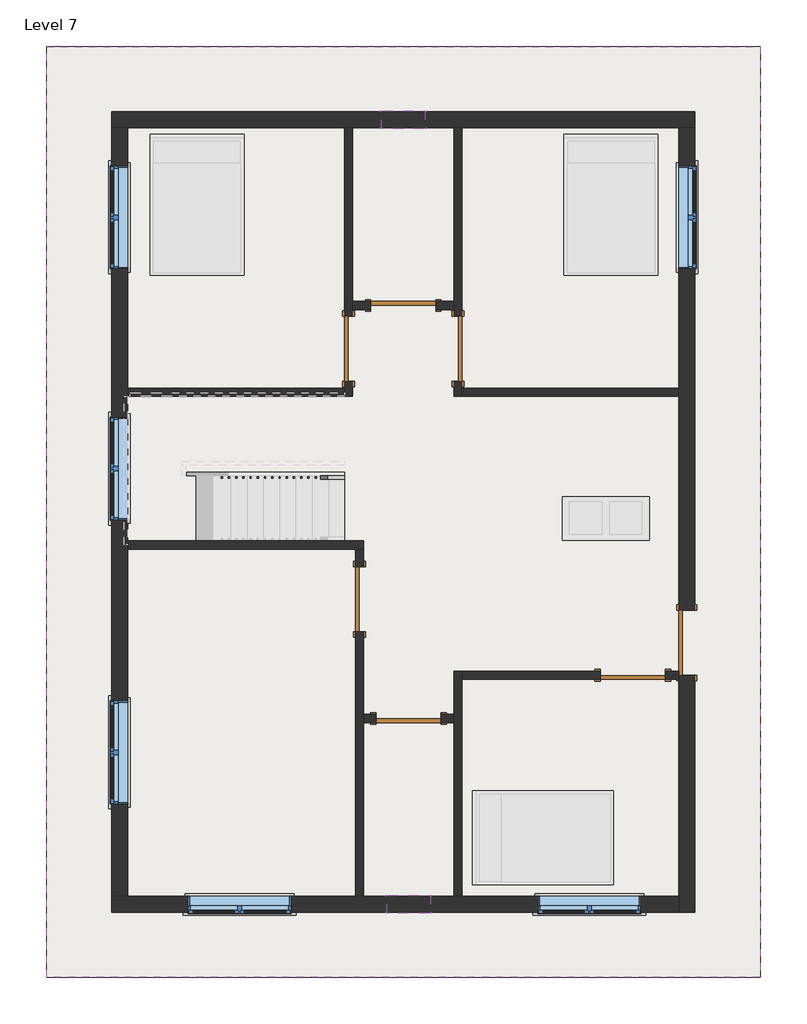
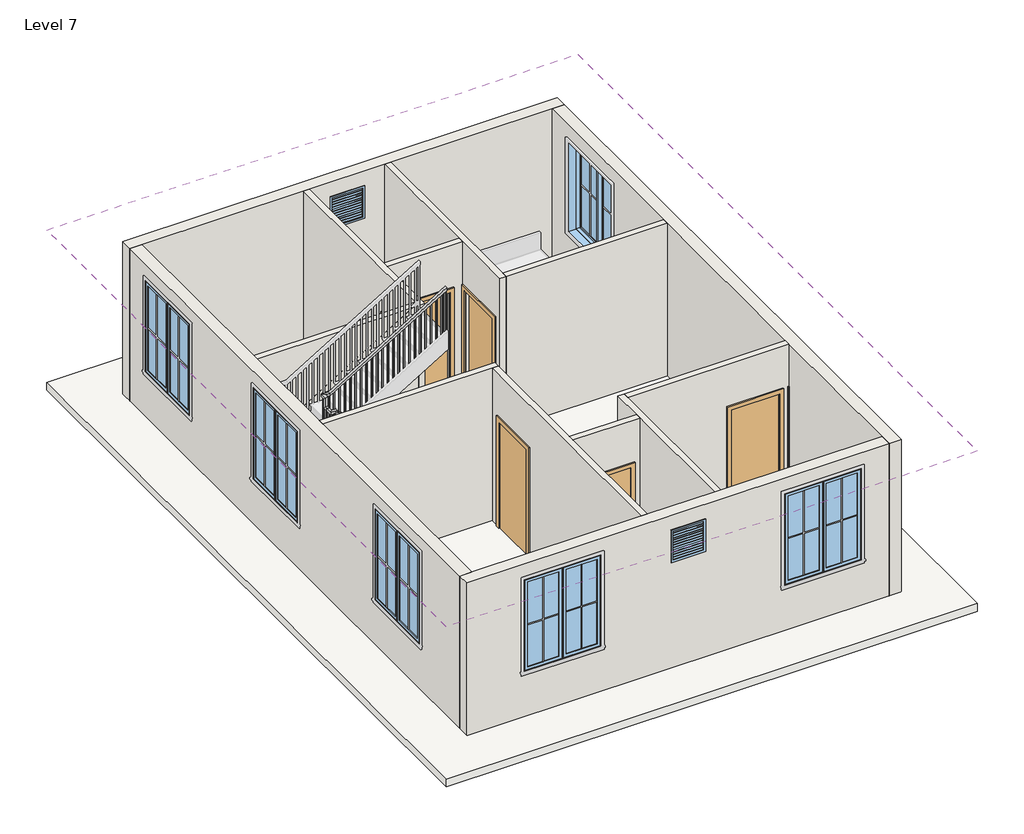
# One storey, part 1 of 2: 14 walls, 8 windows, 7 doors, 2 roofs, 1 railing, 1 slab.
"""IFC4 building model written with IfcOpenShell, lengths in millimetres."""

from ifc_helpers import new_model, si_unit, frame, origin, place, context, project, spatial, polyline, outline, extrude, faceted_brep, transform, mapped, element, save
from components import door_305aa2a5, door_e5f9f3c4, door_0ca8825f, window_9ac97e1a, window_f2d8fef0

model = new_model("IFC4")

# Units and contexts
model_context = context("Model", 3, world=origin())
ifc_project = project(units=[si_unit("LENGTHUNIT", "METRE", prefix="MILLI")], contexts=[model_context])

# Site, building, storey
site = spatial("IfcSite", under=ifc_project)
building = spatial("IfcBuilding", under=site)
storey = spatial("IfcBuildingStorey", under=building, Name="Level 7", Elevation=16002.0)

# Doors
placement = place(None, origin())
door_shape = door_305aa2a5(model_context)
element("IfcDoor", 1, ObjectType="Single-Flush : 36\" x 84\"", at=placement, inside=storey, context=model_context, shape_type="MappedRepresentation", body=[
    mapped(door_shape, transform((-2023.6910855, 2116.5303617, 16002.0), x_axis=(0.0, -1.0, 0.0), y_axis=(1.0, 0.0, 0.0), z_axis=(0.0, 0.0, 1.0))),
])
element("IfcDoor", 2, ObjectType="Single-Flush : 36\" x 84\"", at=placement, inside=storey, context=model_context, shape_type="MappedRepresentation", body=[
    mapped(door_shape, transform((-1179.1410855, -3078.1725945, 16002.0), x_axis=(1.0, 0.0, 0.0), y_axis=(0.0, 1.0, 0.0), z_axis=(0.0, 0.0, 1.0))),
])
element("IfcDoor", 3, ObjectType="Single-Flush : 36\" x 84\"", at=placement, inside=storey, context=model_context, shape_type="MappedRepresentation", body=[
    mapped(door_shape, transform((1970.4589145, -2468.1696383, 16002.0), x_axis=(1.0, 0.0, 0.0), y_axis=(0.0, 1.0, 0.0), z_axis=(0.0, 0.0, 1.0))),
])
door_2_shape = door_e5f9f3c4(model_context)
element("IfcDoor", 4, ObjectType="Single-Flush : 36\" x 84\"", at=placement, inside=storey, context=model_context, shape_type="MappedRepresentation", body=[
    mapped(door_2_shape, transform((-486.9910855, 2116.5303617, 16002.0), x_axis=(0.0, -1.0, 0.0), y_axis=(1.0, 0.0, 0.0), z_axis=(0.0, 0.0, 1.0))),
])
element("IfcDoor", 5, ObjectType="Single-Flush : 36\" x 84\"", at=placement, inside=storey, context=model_context, shape_type="MappedRepresentation", body=[
    mapped(door_2_shape, transform((-1871.2910855, -1401.3696383, 16002.0), x_axis=(0.0, 1.0, 0.0), y_axis=(-1.0, 0.0, 0.0), z_axis=(0.0, 0.0, 1.0))),
])
element("IfcDoor", 6, ObjectType="Single-Flush : 36\" x 84\"", at=placement, inside=storey, context=model_context, shape_type="MappedRepresentation", body=[
    mapped(door_2_shape, transform((-1255.3410855, 2726.1303617, 16002.0), x_axis=(1.0, 0.0, 0.0), y_axis=(0.0, 1.0, 0.0), z_axis=(0.0, 0.0, 1.0))),
])
door_3_shape = door_0ca8825f(model_context)
element("IfcDoor", 7, ObjectType="Single-Flush : 36\" x 84\"", at=placement, inside=storey, context=model_context, shape_type="MappedRepresentation", body=[
    mapped(door_3_shape, transform((2732.4589145, -2010.9696383, 16002.0), x_axis=(0.0, 1.0, 0.0), y_axis=(-1.0, 0.0, 0.0), z_axis=(0.0, 0.0, 1.0))),
])

# Railing
element("IfcRailing", 8, ObjectType="Handrail - Rectangular", at=placement, inside=storey, context=model_context, shape_type="SolidModel", body=[
    faceted_brep([(-2080.8410855, 281.3803617, 17054.9454545), (-2080.8410855, 281.3803617, 16995.5439943), (-2080.8410855, 332.1803617, 16995.5439943), (-2080.8410855, 332.1803617, 17054.9454545), (-4290.6410855, 281.3803617, 18394.2181818), (-4341.4410855, 281.3803617, 18365.6046004), (-4341.4410855, 332.1803617, 18365.6046004), (-4290.6410855, 332.1803617, 18394.2181818), (-4290.6410855, 281.3803617, 18440.4), (-4341.4410855, 281.3803617, 18389.6), (-4341.4410855, 332.1803617, 18389.6), (-4290.6410855, 332.1803617, 18440.4), (-4417.6410855, 281.3803617, 18440.4), (-4417.6410855, 281.3803617, 18389.6), (-4366.8410855, 332.1803617, 18389.6), (-4366.8410855, 332.1803617, 18440.4), (-4417.6410855, 408.3803617, 18440.4), (-4417.6410855, 408.3803617, 18389.6), (-4366.8410855, 408.3803617, 18389.6), (-4366.8410855, 408.3803617, 18440.4), (-4417.6410855, 459.1803617, 18440.4), (-4417.6410855, 509.9803617, 18389.6), (-4366.8410855, 509.9803617, 18389.6), (-4366.8410855, 459.1803617, 18440.4), (-4417.6410855, 459.1803617, 18625.1272727), (-4417.6410855, 509.9803617, 18574.3272727), (-4366.8410855, 509.9803617, 18574.3272727), (-4366.8410855, 459.1803617, 18625.1272727), (-4417.6410855, 586.1803617, 18625.1272727), (-4417.6410855, 586.1803617, 18574.3272727), (-4366.8410855, 535.3803617, 18574.3272727), (-4366.8410855, 535.3803617, 18625.1272727), (-4290.6410855, 586.1803617, 18625.1272727), (-4276.4486761, 586.1803617, 18574.3272727), (-4276.4486761, 535.3803617, 18574.3272727), (-4290.6410855, 535.3803617, 18625.1272727), (-2080.8410855, 586.1803617, 19964.4), (-2080.8410855, 535.3803617, 19964.4), (-2080.8410855, 535.3803617, 19904.9985397), (-2080.8410855, 586.1803617, 19904.9985397)], [[[0, 1, 2, 3]], [[1, 0, 4, 5]], [[2, 1, 5, 6]], [[3, 2, 6, 7]], [[0, 3, 7, 4]], [[5, 4, 8, 9]], [[6, 5, 9, 10]], [[7, 6, 10, 11]], [[4, 7, 11, 8]], [[9, 8, 12, 13]], [[10, 9, 13, 14]], [[11, 10, 14, 15]], [[8, 11, 15, 12]], [[13, 12, 16, 17]], [[14, 13, 17, 18]], [[15, 14, 18, 19]], [[12, 15, 19, 16]], [[17, 16, 20, 21]], [[18, 17, 21, 22]], [[19, 18, 22, 23]], [[16, 19, 23, 20]], [[21, 20, 24, 25]], [[22, 21, 25, 26]], [[23, 22, 26, 27]], [[20, 23, 27, 24]], [[25, 24, 28, 29]], [[26, 25, 29, 30]], [[27, 26, 30, 31]], [[24, 27, 31, 28]], [[29, 28, 32, 33]], [[30, 29, 33, 34]], [[31, 30, 34, 35]], [[28, 31, 35, 32]], [[36, 37, 38, 39]], [[33, 32, 36, 39]], [[34, 33, 39, 38]], [[35, 34, 38, 37]], [[32, 35, 37, 36]]]),
    extrude(outline(polyline([(19864.5894488, -2147.5160855), (19853.0439943, -2166.5660855), (18911.4545455, -2166.5660855), (18911.4545455, -2147.5160855), (19864.5894488, -2147.5160855)])), frame((0.0, 551.2553617, 0.0), z_axis=(0.0, 1.0, 0.0), x_axis=(0.0, 0.0, 1.0)), (0.0, 0.0, 1.0), 19.05),
    extrude(outline(polyline([(19803.0136913, -2249.1160855), (19791.4682367, -2268.1660855), (18911.4545455, -2268.1660855), (18911.4545455, -2249.1160855), (19803.0136913, -2249.1160855)])), frame((0.0, 551.2553617, 0.0), z_axis=(0.0, 1.0, 0.0), x_axis=(0.0, 0.0, 1.0)), (0.0, 0.0, 1.0), 19.05),
    extrude(outline(polyline([(19741.4379337, -2350.7160855), (19729.8924791, -2369.7660855), (18772.9090909, -2369.7660855), (18772.9090909, -2350.7160855), (19741.4379337, -2350.7160855)])), frame((0.0, 551.2553617, 0.0), z_axis=(0.0, 1.0, 0.0), x_axis=(0.0, 0.0, 1.0)), (0.0, 0.0, 1.0), 19.05),
    extrude(outline(polyline([(19679.8621761, -2452.3160855), (19668.3167216, -2471.3660855), (18772.9090909, -2471.3660855), (18772.9090909, -2452.3160855), (19679.8621761, -2452.3160855)])), frame((0.0, 551.2553617, 0.0), z_axis=(0.0, 1.0, 0.0), x_axis=(0.0, 0.0, 1.0)), (0.0, 0.0, 1.0), 19.05),
    extrude(outline(polyline([(19618.2864185, -2553.9160855), (19606.740964, -2572.9660855), (18634.3636364, -2572.9660855), (18634.3636364, -2553.9160855), (19618.2864185, -2553.9160855)])), frame((0.0, 551.2553617, 0.0), z_axis=(0.0, 1.0, 0.0), x_axis=(0.0, 0.0, 1.0)), (0.0, 0.0, 1.0), 19.05),
    extrude(outline(polyline([(19556.710661, -2655.5160855), (19545.1652064, -2674.5660855), (18634.3636364, -2674.5660855), (18634.3636364, -2655.5160855), (19556.710661, -2655.5160855)])), frame((0.0, 551.2553617, 0.0), z_axis=(0.0, 1.0, 0.0), x_axis=(0.0, 0.0, 1.0)), (0.0, 0.0, 1.0), 19.05),
    extrude(outline(polyline([(19495.1349034, -2757.1160855), (19483.5894488, -2776.1660855), (18634.3636364, -2776.1660855), (18634.3636364, -2757.1160855), (19495.1349034, -2757.1160855)])), frame((0.0, 551.2553617, 0.0), z_axis=(0.0, 1.0, 0.0), x_axis=(0.0, 0.0, 1.0)), (0.0, 0.0, 1.0), 19.05),
    extrude(outline(polyline([(19433.5591458, -2858.7160855), (19422.0136913, -2877.7660855), (18495.8181818, -2877.7660855), (18495.8181818, -2858.7160855), (19433.5591458, -2858.7160855)])), frame((0.0, 551.2553617, 0.0), z_axis=(0.0, 1.0, 0.0), x_axis=(0.0, 0.0, 1.0)), (0.0, 0.0, 1.0), 19.05),
    extrude(outline(polyline([(19371.9833882, -2960.3160855), (19360.4379337, -2979.3660855), (18495.8181818, -2979.3660855), (18495.8181818, -2960.3160855), (19371.9833882, -2960.3160855)])), frame((0.0, 551.2553617, 0.0), z_axis=(0.0, 1.0, 0.0), x_axis=(0.0, 0.0, 1.0)), (0.0, 0.0, 1.0), 19.05),
    extrude(outline(polyline([(19310.4076307, -3061.9160855), (19298.8621761, -3080.9660855), (18357.2727273, -3080.9660855), (18357.2727273, -3061.9160855), (19310.4076307, -3061.9160855)])), frame((0.0, 551.2553617, 0.0), z_axis=(0.0, 1.0, 0.0), x_axis=(0.0, 0.0, 1.0)), (0.0, 0.0, 1.0), 19.05),
    extrude(outline(polyline([(19248.8318731, -3163.5160855), (19237.2864185, -3182.5660855), (18357.2727273, -3182.5660855), (18357.2727273, -3163.5160855), (19248.8318731, -3163.5160855)])), frame((0.0, 551.2553617, 0.0), z_axis=(0.0, 1.0, 0.0), x_axis=(0.0, 0.0, 1.0)), (0.0, 0.0, 1.0), 19.05),
    extrude(outline(polyline([(19187.2561155, -3265.1160855), (19175.710661, -3284.1660855), (18218.7272727, -3284.1660855), (18218.7272727, -3265.1160855), (19187.2561155, -3265.1160855)])), frame((0.0, 551.2553617, 0.0), z_axis=(0.0, 1.0, 0.0), x_axis=(0.0, 0.0, 1.0)), (0.0, 0.0, 1.0), 19.05),
    extrude(outline(polyline([(19125.6803579, -3366.7160855), (19114.1349034, -3385.7660855), (18218.7272727, -3385.7660855), (18218.7272727, -3366.7160855), (19125.6803579, -3366.7160855)])), frame((0.0, 551.2553617, 0.0), z_axis=(0.0, 1.0, 0.0), x_axis=(0.0, 0.0, 1.0)), (0.0, 0.0, 1.0), 19.05),
    extrude(outline(polyline([(19064.1046004, -3468.3160855), (19052.5591458, -3487.3660855), (18080.1818182, -3487.3660855), (18080.1818182, -3468.3160855), (19064.1046004, -3468.3160855)])), frame((0.0, 551.2553617, 0.0), z_axis=(0.0, 1.0, 0.0), x_axis=(0.0, 0.0, 1.0)), (0.0, 0.0, 1.0), 19.05),
    extrude(outline(polyline([(19002.5288428, -3569.9160855), (18990.9833882, -3588.9660855), (18080.1818182, -3588.9660855), (18080.1818182, -3569.9160855), (19002.5288428, -3569.9160855)])), frame((0.0, 551.2553617, 0.0), z_axis=(0.0, 1.0, 0.0), x_axis=(0.0, 0.0, 1.0)), (0.0, 0.0, 1.0), 19.05),
    extrude(outline(polyline([(18940.9530852, -3671.5160855), (18929.4076307, -3690.5660855), (18080.1818182, -3690.5660855), (18080.1818182, -3671.5160855), (18940.9530852, -3671.5160855)])), frame((0.0, 551.2553617, 0.0), z_axis=(0.0, 1.0, 0.0), x_axis=(0.0, 0.0, 1.0)), (0.0, 0.0, 1.0), 19.05),
    extrude(outline(polyline([(18879.3773276, -3773.1160855), (18867.8318731, -3792.1660855), (17941.6363636, -3792.1660855), (17941.6363636, -3773.1160855), (18879.3773276, -3773.1160855)])), frame((0.0, 551.2553617, 0.0), z_axis=(0.0, 1.0, 0.0), x_axis=(0.0, 0.0, 1.0)), (0.0, 0.0, 1.0), 19.05),
    extrude(outline(polyline([(18817.80157, -3874.7160855), (18806.2561155, -3893.7660855), (17941.6363636, -3893.7660855), (17941.6363636, -3874.7160855), (18817.80157, -3874.7160855)])), frame((0.0, 551.2553617, 0.0), z_axis=(0.0, 1.0, 0.0), x_axis=(0.0, 0.0, 1.0)), (0.0, 0.0, 1.0), 19.05),
    extrude(outline(polyline([(18756.2258125, -3976.3160855), (18744.6803579, -3995.3660855), (17803.0909091, -3995.3660855), (17803.0909091, -3976.3160855), (18756.2258125, -3976.3160855)])), frame((0.0, 551.2553617, 0.0), z_axis=(0.0, 1.0, 0.0), x_axis=(0.0, 0.0, 1.0)), (0.0, 0.0, 1.0), 19.05),
    extrude(outline(polyline([(18694.6500549, -4077.9160855), (18683.1046004, -4096.9660855), (17803.0909091, -4096.9660855), (17803.0909091, -4077.9160855), (18694.6500549, -4077.9160855)])), frame((0.0, 551.2553617, 0.0), z_axis=(0.0, 1.0, 0.0), x_axis=(0.0, 0.0, 1.0)), (0.0, 0.0, 1.0), 19.05),
    extrude(outline(polyline([(18633.0742973, -4179.5160855), (18621.5288428, -4198.5660855), (17664.5454545, -4198.5660855), (17664.5454545, -4179.5160855), (18633.0742973, -4179.5160855)])), frame((0.0, 551.2553617, 0.0), z_axis=(0.0, 1.0, 0.0), x_axis=(0.0, 0.0, 1.0)), (0.0, 0.0, 1.0), 19.05),
    extrude(outline(polyline([(18571.4985397, -4281.1160855), (18559.9530852, -4300.1660855), (17664.5454545, -4300.1660855), (17664.5454545, -4281.1160855), (18571.4985397, -4281.1160855)])), frame((0.0, 551.2553617, 0.0), z_axis=(0.0, 1.0, 0.0), x_axis=(0.0, 0.0, 1.0)), (0.0, 0.0, 1.0), 19.05),
    extrude(outline(polyline([(-4382.7160855, 500.4553617), (-4401.7660855, 500.4553617), (-4401.7660855, 519.5053617), (-4382.7160855, 519.5053617), (-4382.7160855, 500.4553617)])), frame((0.0, 0.0, 17526.0), z_axis=(0.0, 0.0, 1.0), x_axis=(1.0, 0.0, 0.0)), (0.0, 0.0, 1.0), 1048.3272727),
    extrude(outline(polyline([(-4382.7160855, 398.8553617), (-4401.7660855, 398.8553617), (-4401.7660855, 417.9053617), (-4382.7160855, 417.9053617), (-4382.7160855, 398.8553617)])), frame((0.0, 0.0, 17526.0), z_axis=(0.0, 0.0, 1.0), x_axis=(1.0, 0.0, 0.0)), (0.0, 0.0, 1.0), 863.6),
    extrude(outline(polyline([(-4306.5160855, 316.3053617), (-4306.5160855, 297.2553617), (-4325.5660855, 297.2553617), (-4325.5660855, 316.3053617), (-4306.5160855, 316.3053617)])), frame((0.0, 0.0, 17387.4545455), z_axis=(0.0, 0.0, 1.0), x_axis=(1.0, 0.0, 0.0)), (0.0, 0.0, 1.0), 1002.1454545),
    extrude(outline(polyline([(18282.8621761, -4204.9160855), (18294.4076307, -4223.9660855), (17387.4545455, -4223.9660855), (17387.4545455, -4204.9160855), (18282.8621761, -4204.9160855)])), frame((0.0, 297.2553617, 0.0), z_axis=(0.0, 1.0, 0.0), x_axis=(0.0, 0.0, 1.0)), (0.0, 0.0, 1.0), 19.05),
    extrude(outline(polyline([(18221.2864185, -4103.3160855), (18232.8318731, -4122.3660855), (17248.9090909, -4122.3660855), (17248.9090909, -4103.3160855), (18221.2864185, -4103.3160855)])), frame((0.0, 297.2553617, 0.0), z_axis=(0.0, 1.0, 0.0), x_axis=(0.0, 0.0, 1.0)), (0.0, 0.0, 1.0), 19.05),
    extrude(outline(polyline([(18159.710661, -4001.7160855), (18171.2561155, -4020.7660855), (17248.9090909, -4020.7660855), (17248.9090909, -4001.7160855), (18159.710661, -4001.7160855)])), frame((0.0, 297.2553617, 0.0), z_axis=(0.0, 1.0, 0.0), x_axis=(0.0, 0.0, 1.0)), (0.0, 0.0, 1.0), 19.05),
    extrude(outline(polyline([(18098.1349034, -3900.1160855), (18109.6803579, -3919.1660855), (17248.9090909, -3919.1660855), (17248.9090909, -3900.1160855), (18098.1349034, -3900.1160855)])), frame((0.0, 297.2553617, 0.0), z_axis=(0.0, 1.0, 0.0), x_axis=(0.0, 0.0, 1.0)), (0.0, 0.0, 1.0), 19.05),
    extrude(outline(polyline([(18036.5591458, -3798.5160855), (18048.1046004, -3817.5660855), (17110.3636364, -3817.5660855), (17110.3636364, -3798.5160855), (18036.5591458, -3798.5160855)])), frame((0.0, 297.2553617, 0.0), z_axis=(0.0, 1.0, 0.0), x_axis=(0.0, 0.0, 1.0)), (0.0, 0.0, 1.0), 19.05),
    extrude(outline(polyline([(17974.9833882, -3696.9160855), (17986.5288428, -3715.9660855), (17110.3636364, -3715.9660855), (17110.3636364, -3696.9160855), (17974.9833882, -3696.9160855)])), frame((0.0, 297.2553617, 0.0), z_axis=(0.0, 1.0, 0.0), x_axis=(0.0, 0.0, 1.0)), (0.0, 0.0, 1.0), 19.05),
    extrude(outline(polyline([(17913.4076307, -3595.3160855), (17924.9530852, -3614.3660855), (16971.8181818, -3614.3660855), (16971.8181818, -3595.3160855), (17913.4076307, -3595.3160855)])), frame((0.0, 297.2553617, 0.0), z_axis=(0.0, 1.0, 0.0), x_axis=(0.0, 0.0, 1.0)), (0.0, 0.0, 1.0), 19.05),
    extrude(outline(polyline([(17851.8318731, -3493.7160855), (17863.3773276, -3512.7660855), (16971.8181818, -3512.7660855), (16971.8181818, -3493.7160855), (17851.8318731, -3493.7160855)])), frame((0.0, 297.2553617, 0.0), z_axis=(0.0, 1.0, 0.0), x_axis=(0.0, 0.0, 1.0)), (0.0, 0.0, 1.0), 19.05),
    extrude(outline(polyline([(17790.2561155, -3392.1160855), (17801.80157, -3411.1660855), (16833.2727273, -3411.1660855), (16833.2727273, -3392.1160855), (17790.2561155, -3392.1160855)])), frame((0.0, 297.2553617, 0.0), z_axis=(0.0, 1.0, 0.0), x_axis=(0.0, 0.0, 1.0)), (0.0, 0.0, 1.0), 19.05),
    extrude(outline(polyline([(17728.6803579, -3290.5160855), (17740.2258125, -3309.5660855), (16833.2727273, -3309.5660855), (16833.2727273, -3290.5160855), (17728.6803579, -3290.5160855)])), frame((0.0, 297.2553617, 0.0), z_axis=(0.0, 1.0, 0.0), x_axis=(0.0, 0.0, 1.0)), (0.0, 0.0, 1.0), 19.05),
    extrude(outline(polyline([(17667.1046004, -3188.9160855), (17678.6500549, -3207.9660855), (16694.7272727, -3207.9660855), (16694.7272727, -3188.9160855), (17667.1046004, -3188.9160855)])), frame((0.0, 297.2553617, 0.0), z_axis=(0.0, 1.0, 0.0), x_axis=(0.0, 0.0, 1.0)), (0.0, 0.0, 1.0), 19.05),
    extrude(outline(polyline([(17605.5288428, -3087.3160855), (17617.0742973, -3106.3660855), (16694.7272727, -3106.3660855), (16694.7272727, -3087.3160855), (17605.5288428, -3087.3160855)])), frame((0.0, 297.2553617, 0.0), z_axis=(0.0, 1.0, 0.0), x_axis=(0.0, 0.0, 1.0)), (0.0, 0.0, 1.0), 19.05),
    extrude(outline(polyline([(17543.9530852, -2985.7160855), (17555.4985397, -3004.7660855), (16694.7272727, -3004.7660855), (16694.7272727, -2985.7160855), (17543.9530852, -2985.7160855)])), frame((0.0, 297.2553617, 0.0), z_axis=(0.0, 1.0, 0.0), x_axis=(0.0, 0.0, 1.0)), (0.0, 0.0, 1.0), 19.05),
    extrude(outline(polyline([(17482.3773276, -2884.1160855), (17493.9227822, -2903.1660855), (16556.1818182, -2903.1660855), (16556.1818182, -2884.1160855), (17482.3773276, -2884.1160855)])), frame((0.0, 297.2553617, 0.0), z_axis=(0.0, 1.0, 0.0), x_axis=(0.0, 0.0, 1.0)), (0.0, 0.0, 1.0), 19.05),
    extrude(outline(polyline([(17420.80157, -2782.5160855), (17432.3470246, -2801.5660855), (16556.1818182, -2801.5660855), (16556.1818182, -2782.5160855), (17420.80157, -2782.5160855)])), frame((0.0, 297.2553617, 0.0), z_axis=(0.0, 1.0, 0.0), x_axis=(0.0, 0.0, 1.0)), (0.0, 0.0, 1.0), 19.05),
    extrude(outline(polyline([(17359.2258125, -2680.9160855), (17370.771267, -2699.9660855), (16417.6363636, -2699.9660855), (16417.6363636, -2680.9160855), (17359.2258125, -2680.9160855)])), frame((0.0, 297.2553617, 0.0), z_axis=(0.0, 1.0, 0.0), x_axis=(0.0, 0.0, 1.0)), (0.0, 0.0, 1.0), 19.05),
    extrude(outline(polyline([(17297.6500549, -2579.3160855), (17309.1955094, -2598.3660855), (16417.6363636, -2598.3660855), (16417.6363636, -2579.3160855), (17297.6500549, -2579.3160855)])), frame((0.0, 297.2553617, 0.0), z_axis=(0.0, 1.0, 0.0), x_axis=(0.0, 0.0, 1.0)), (0.0, 0.0, 1.0), 19.05),
    extrude(outline(polyline([(17236.0742973, -2477.7160855), (17247.6197519, -2496.7660855), (16279.0909091, -2496.7660855), (16279.0909091, -2477.7160855), (17236.0742973, -2477.7160855)])), frame((0.0, 297.2553617, 0.0), z_axis=(0.0, 1.0, 0.0), x_axis=(0.0, 0.0, 1.0)), (0.0, 0.0, 1.0), 19.05),
    extrude(outline(polyline([(17174.4985397, -2376.1160855), (17186.0439943, -2395.1660855), (16279.0909091, -2395.1660855), (16279.0909091, -2376.1160855), (17174.4985397, -2376.1160855)])), frame((0.0, 297.2553617, 0.0), z_axis=(0.0, 1.0, 0.0), x_axis=(0.0, 0.0, 1.0)), (0.0, 0.0, 1.0), 19.05),
    extrude(outline(polyline([(17112.9227822, -2274.5160855), (17124.4682367, -2293.5660855), (16140.5454545, -2293.5660855), (16140.5454545, -2274.5160855), (17112.9227822, -2274.5160855)])), frame((0.0, 297.2553617, 0.0), z_axis=(0.0, 1.0, 0.0), x_axis=(0.0, 0.0, 1.0)), (0.0, 0.0, 1.0), 19.05),
    extrude(outline(polyline([(17051.3470246, -2172.9160855), (17062.8924791, -2191.9660855), (16140.5454545, -2191.9660855), (16140.5454545, -2172.9160855), (17051.3470246, -2172.9160855)])), frame((0.0, 297.2553617, 0.0), z_axis=(0.0, 1.0, 0.0), x_axis=(0.0, 0.0, 1.0)), (0.0, 0.0, 1.0), 19.05),
    extrude(outline(polyline([(-4382.7160855, 551.2553617), (-4401.7660855, 551.2553617), (-4401.7660855, 570.3053617), (-4382.7160855, 570.3053617), (-4382.7160855, 551.2553617)])), frame((0.0, 0.0, 17526.0), z_axis=(0.0, 0.0, 1.0), x_axis=(1.0, 0.0, 0.0)), (0.0, 0.0, 1.0), 1048.3272727),
    extrude(outline(polyline([(-4382.7160855, 316.3053617), (-4382.7160855, 297.2553617), (-4401.7660855, 297.2553617), (-4401.7660855, 316.3053617), (-4382.7160855, 316.3053617)])), frame((0.0, 0.0, 17526.0), z_axis=(0.0, 0.0, 1.0), x_axis=(1.0, 0.0, 0.0)), (0.0, 0.0, 1.0), 863.6),
    extrude(outline(polyline([(19904.9985397, -2080.8410855), (19893.4530852, -2099.8910855), (18911.4545455, -2099.8910855), (18911.4545455, -2080.8410855), (19904.9985397, -2080.8410855)])), frame((0.0, 551.2553617, 0.0), z_axis=(0.0, 1.0, 0.0), x_axis=(0.0, 0.0, 1.0)), (0.0, 0.0, 1.0), 19.05),
    extrude(outline(polyline([(16995.5439943, -2080.8410855), (17007.0894488, -2099.8910855), (16140.5454545, -2099.8910855), (16140.5454545, -2080.8410855), (16995.5439943, -2080.8410855)])), frame((0.0, 297.2553617, 0.0), z_axis=(0.0, 1.0, 0.0), x_axis=(0.0, 0.0, 1.0)), (0.0, 0.0, 1.0), 19.05),
])

# Roofs
element("IfcRoof", 9, ObjectType="ROOF 6\"", at=placement, inside=storey, context=model_context, shape_type="SweptSolid", body=[
    extrude(outline(polyline([(-6271.8410855, 6364.6803617), (3761.1589145, 6364.6803617), (3761.1589145, -6716.3196383), (-6271.8410855, -6716.3196383), (-6271.8410855, 6364.6803617)])), frame((0.0, 0.0, 15849.6), z_axis=(0.0, 0.0, 1.0), x_axis=(1.0, 0.0, 0.0)), (0.0, 0.0, 1.0), 152.4),
])
element("IfcRoof", 10, ObjectType="ROOF 6\"", at=placement, inside=storey, context=model_context, shape_type="SweptSolid", body=[
    extrude(outline(polyline([(-6271.8410855, 6364.6803617), (3761.1589145, 6364.6803617), (3761.1589145, -6716.3196383), (-6271.8410855, -6716.3196383), (-6271.8410855, 6364.6803617)])), frame((0.0, 0.0, 19050.0), z_axis=(0.0, 0.0, 1.0), x_axis=(1.0, 0.0, 0.0)), (0.0, 0.0, 1.0), 152.4),
])

# Slab
element("IfcSlab", 11, ObjectType="FLOOR 6\"", at=placement, inside=storey, context=model_context, shape_type="SweptSolid", body=[
    extrude(outline(polyline([(2846.7589145, 5450.2803617), (2846.7589145, -5801.9196383), (-5357.4410855, -5801.9196383), (-5357.4410855, 5450.2803617), (2846.7589145, 5450.2803617)])), frame((0.0, 0.0, 15849.6), z_axis=(0.0, 0.0, 1.0), x_axis=(1.0, 0.0, 0.0)), (0.0, 0.0, 1.0), 152.4),
])

# Walls
element("IfcWall", 12, ObjectType="WALL 4.5\"", at=placement, inside=storey, context=model_context, shape_type="Brep", body=[
    faceted_brep([(-2080.8410855, 1659.3303617, 18135.6), (-2080.8410855, 1659.3303617, 16002.0), (-2080.8410855, 1564.0803617, 16002.0), (-2080.8410855, 1449.7803617, 16002.0), (-2080.8410855, 1449.7803617, 19050.0), (-2080.8410855, 1564.0803617, 19050.0), (-2080.8410855, 5221.6803617, 19050.0), (-2080.8410855, 5221.6803617, 16002.0), (-2080.8410855, 2573.7303617, 16002.0), (-2080.8410855, 2573.7303617, 18135.6), (-1966.5410855, 1449.7803617, 16002.0), (-1966.5410855, 1659.3303617, 16002.0), (-1966.5410855, 1659.3303617, 18135.6), (-1966.5410855, 2573.7303617, 18135.6), (-1966.5410855, 2573.7303617, 16002.0), (-1966.5410855, 2668.9803617, 16002.0), (-1966.5410855, 2783.2803617, 16002.0), (-1966.5410855, 5221.6803617, 16002.0), (-1966.5410855, 5221.6803617, 19050.0), (-1966.5410855, 2783.2803617, 19050.0), (-1966.5410855, 2668.9803617, 19050.0), (-1966.5410855, 1449.7803617, 19050.0)], [[[0, 1, 2, 3, 4, 5, 6, 7, 8, 9]], [[10, 11, 12, 13, 14, 15, 16, 17, 18, 19, 20, 21]], [[8, 7, 17, 16, 15, 14]], [[3, 2, 1, 11, 10]], [[7, 6, 18, 17]], [[4, 3, 10, 21]], [[12, 11, 1, 0]], [[13, 12, 0, 9]], [[14, 13, 9, 8]], [[6, 5, 4, 21, 20, 19, 18]]]),
])
element("IfcWall", 13, ObjectType="WALL 4.5\"", at=placement, inside=storey, context=model_context, shape_type="SweptSolid", body=[
    extrude(outline(polyline([(-5128.8410855, 1564.0803617), (-2080.8410855, 1564.0803617), (-2080.8410855, 1449.7803617), (-5128.8410855, 1449.7803617), (-5128.8410855, 1564.0803617)])), frame((0.0, 0.0, 16002.0), z_axis=(0.0, 0.0, 1.0), x_axis=(1.0, 0.0, 0.0)), (0.0, 0.0, 1.0), 3048.0),
])
element("IfcWall", 14, ObjectType="WALL 4.5\"", at=placement, inside=storey, context=model_context, shape_type="Brep", body=[
    faceted_brep([(-544.1410855, 1659.3303617, 18135.6), (-544.1410855, 1659.3303617, 16002.0), (-544.1410855, 1449.7803617, 16002.0), (-544.1410855, 1449.7803617, 19050.0), (-544.1410855, 2668.9803617, 19050.0), (-544.1410855, 2783.2803617, 19050.0), (-544.1410855, 5221.6803617, 19050.0), (-544.1410855, 5221.6803617, 16002.0), (-544.1410855, 2783.2803617, 16002.0), (-544.1410855, 2668.9803617, 16002.0), (-544.1410855, 2573.7303617, 16002.0), (-544.1410855, 2573.7303617, 18135.6), (-429.8410855, 1449.7803617, 16002.0), (-429.8410855, 1564.0803617, 16002.0), (-429.8410855, 1659.3303617, 16002.0), (-429.8410855, 1659.3303617, 18135.6), (-429.8410855, 2573.7303617, 18135.6), (-429.8410855, 2573.7303617, 16002.0), (-429.8410855, 5221.6803617, 16002.0), (-429.8410855, 5221.6803617, 19050.0), (-429.8410855, 1564.0803617, 19050.0), (-429.8410855, 1449.7803617, 19050.0)], [[[0, 1, 2, 3, 4, 5, 6, 7, 8, 9, 10, 11]], [[12, 13, 14, 15, 16, 17, 18, 19, 20, 21]], [[2, 1, 14, 13, 12]], [[10, 9, 8, 7, 18, 17]], [[7, 6, 19, 18]], [[3, 2, 12, 21]], [[15, 14, 1, 0]], [[16, 15, 0, 11]], [[17, 16, 11, 10]], [[6, 5, 4, 3, 21, 20, 19]]]),
])
element("IfcWall", 15, ObjectType="WALL 4.5\"", at=placement, inside=storey, context=model_context, shape_type="SweptSolid", body=[
    extrude(outline(polyline([(2618.1589145, 1449.7803617), (-429.8410855, 1449.7803617), (-429.8410855, 1564.0803617), (2618.1589145, 1564.0803617), (2618.1589145, 1449.7803617)])), frame((0.0, 0.0, 16002.0), z_axis=(0.0, 0.0, 1.0), x_axis=(1.0, 0.0, 0.0)), (0.0, 0.0, 1.0), 3048.0),
])
element("IfcWall", 16, ObjectType="WALL 4.5\"", at=placement, inside=storey, context=model_context, shape_type="Brep", body=[
    faceted_brep([(-5128.8410855, -696.5196383, 16002.0), (-1928.4410855, -696.5196383, 16002.0), (-1814.1410855, -696.5196383, 16002.0), (-1814.1410855, -696.5196383, 19050.0), (-1928.4410855, -696.5196383, 19050.0), (-5128.8410855, -696.5196383, 19050.0), (-5128.8410855, -582.2196383, 16002.0), (-5128.8410855, -582.2196383, 19050.0), (-1814.1410855, -582.2196383, 19050.0), (-1814.1410855, -582.2196383, 16002.0)], [[[0, 1, 2, 3, 4, 5]], [[6, 7, 8, 9]], [[2, 1, 0, 6, 9]], [[0, 5, 7, 6]], [[3, 2, 9, 8]], [[5, 4, 3, 8, 7]]]),
])
element("IfcWall", 17, ObjectType="WALL 4.5\"", at=placement, inside=storey, context=model_context, shape_type="Brep", body=[
    faceted_brep([(-1814.1410855, -944.1696383, 18135.6), (-1814.1410855, -944.1696383, 16002.0), (-1814.1410855, -696.5196383, 16002.0), (-1814.1410855, -696.5196383, 19050.0), (-1814.1410855, -3021.0225945, 19050.0), (-1814.1410855, -3135.3225945, 19050.0), (-1814.1410855, -5573.3196383, 19050.0), (-1814.1410855, -5573.3196383, 16002.0), (-1814.1410855, -3135.3225945, 16002.0), (-1814.1410855, -3021.0225945, 16002.0), (-1814.1410855, -1858.5696383, 16002.0), (-1814.1410855, -1858.5696383, 18135.6), (-1928.4410855, -696.5196383, 16002.0), (-1928.4410855, -944.1696383, 16002.0), (-1928.4410855, -944.1696383, 18135.6), (-1928.4410855, -1858.5696383, 18135.6), (-1928.4410855, -1858.5696383, 16002.0), (-1928.4410855, -5573.3196383, 16002.0), (-1928.4410855, -5573.3196383, 19050.0), (-1928.4410855, -696.5196383, 19050.0)], [[[0, 1, 2, 3, 4, 5, 6, 7, 8, 9, 10, 11]], [[12, 13, 14, 15, 16, 17, 18, 19]], [[2, 1, 13, 12]], [[10, 9, 8, 7, 17, 16]], [[3, 2, 12, 19]], [[7, 6, 18, 17]], [[14, 13, 1, 0]], [[15, 14, 0, 11]], [[16, 15, 11, 10]], [[6, 5, 4, 3, 19, 18]]]),
])
element("IfcWall", 18, ObjectType="WALL 4.5\"", at=placement, inside=storey, context=model_context, shape_type="SweptSolid", body=[
    extrude(outline(polyline([(18135.6, -721.9410855), (16002.0, -721.9410855), (16002.0, -544.1410855), (19050.0, -544.1410855), (19050.0, -1814.1410855), (16002.0, -1814.1410855), (16002.0, -1636.3410855), (18135.6, -1636.3410855), (18135.6, -721.9410855)])), frame((0.0, -3135.3225945, 0.0), z_axis=(0.0, 1.0, 0.0), x_axis=(0.0, 0.0, 1.0)), (0.0, 0.0, 1.0), 114.3),
])
element("IfcWall", 19, ObjectType="WALL 4.5\"", at=placement, inside=storey, context=model_context, shape_type="Brep", body=[
    faceted_brep([(-544.1410855, -2411.0196383, 16002.0), (-544.1410855, -3021.0225945, 16002.0), (-544.1410855, -3135.3225945, 16002.0), (-544.1410855, -5573.3196383, 16002.0), (-544.1410855, -5573.3196383, 19050.0), (-544.1410855, -3135.3225945, 19050.0), (-544.1410855, -3021.0225945, 19050.0), (-544.1410855, -2411.0196383, 19050.0), (-429.8410855, -2411.0196383, 16002.0), (-429.8410855, -2411.0196383, 19050.0), (-429.8410855, -2525.3196383, 19050.0), (-429.8410855, -5573.3196383, 19050.0), (-429.8410855, -5573.3196383, 16002.0), (-429.8410855, -2525.3196383, 16002.0)], [[[0, 1, 2, 3, 4, 5, 6, 7]], [[8, 9, 10, 11, 12, 13]], [[3, 2, 1, 0, 8, 13, 12]], [[4, 3, 12, 11]], [[0, 7, 9, 8]], [[7, 6, 5, 4, 11, 10, 9]]]),
])
element("IfcWall", 20, ObjectType="WALL 4.5\"", at=placement, inside=storey, context=model_context, shape_type="Brep", body=[
    faceted_brep([(2427.6589145, -2525.3196383, 18135.6), (2427.6589145, -2525.3196383, 16002.0), (2618.1589145, -2525.3196383, 16002.0), (2618.1589145, -2525.3196383, 19050.0), (-429.8410855, -2525.3196383, 19050.0), (-429.8410855, -2525.3196383, 16002.0), (1513.2589145, -2525.3196383, 16002.0), (1513.2589145, -2525.3196383, 18135.6), (2618.1589145, -2411.0196383, 16002.0), (2427.6589145, -2411.0196383, 16002.0), (2427.6589145, -2411.0196383, 18135.6), (1513.2589145, -2411.0196383, 18135.6), (1513.2589145, -2411.0196383, 16002.0), (-429.8410855, -2411.0196383, 16002.0), (-429.8410855, -2411.0196383, 19050.0), (2618.1589145, -2411.0196383, 19050.0), (2618.1589145, -2468.1696383, 16002.0)], [[[0, 1, 2, 3, 4, 5, 6, 7]], [[8, 9, 10, 11, 12, 13, 14, 15]], [[6, 5, 13, 12]], [[2, 1, 9, 8, 16]], [[5, 4, 14, 13]], [[3, 2, 16, 8, 15]], [[10, 9, 1, 0]], [[11, 10, 0, 7]], [[12, 11, 7, 6]], [[4, 3, 15, 14]]]),
])
element("IfcWall", 21, ObjectType="WALL 4.5\"", at=placement, inside=storey, context=model_context, shape_type="SweptSolid", body=[
    extrude(outline(polyline([(18135.6, -798.1410855), (16002.0, -798.1410855), (16002.0, -544.1410855), (19050.0, -544.1410855), (19050.0, -1966.5410855), (16002.0, -1966.5410855), (16002.0, -1712.5410855), (18135.6, -1712.5410855), (18135.6, -798.1410855)])), frame((0.0, 2668.9803617, 0.0), z_axis=(0.0, 1.0, 0.0), x_axis=(0.0, 0.0, 1.0)), (0.0, 0.0, 1.0), 114.3),
])
element("IfcWall", 22, ObjectType="WALL 9\"", at=placement, inside=storey, context=model_context, shape_type="Brep", body=[
    faceted_brep([(-5357.4410855, 5221.6803617, 16002.0), (-5128.8410855, 5221.6803617, 16002.0), (-2080.8410855, 5221.6803617, 16002.0), (-1966.5410855, 5221.6803617, 16002.0), (-544.1410855, 5221.6803617, 16002.0), (-429.8410855, 5221.6803617, 16002.0), (2618.1589145, 5221.6803617, 16002.0), (2846.7589145, 5221.6803617, 16002.0), (2846.7589145, 5221.6803617, 19050.0), (2618.1589145, 5221.6803617, 19050.0), (-429.8410855, 5221.6803617, 19050.0), (-544.1410855, 5221.6803617, 19050.0), (-1966.5410855, 5221.6803617, 19050.0), (-2080.8410855, 5221.6803617, 19050.0), (-5128.8410855, 5221.6803617, 19050.0), (-5357.4410855, 5221.6803617, 19050.0), (-950.5410855, 5221.6803617, 18745.2), (-950.5410855, 5221.6803617, 18135.6), (-1560.1410855, 5221.6803617, 18135.6), (-1560.1410855, 5221.6803617, 18745.2), (-5357.4410855, 5450.2803617, 16002.0), (-5357.4410855, 5450.2803617, 19050.0), (2846.7589145, 5450.2803617, 19050.0), (2846.7589145, 5450.2803617, 16002.0), (-950.5410855, 5450.2803617, 18745.2), (-1560.1410855, 5450.2803617, 18745.2), (-1560.1410855, 5450.2803617, 18135.6), (-950.5410855, 5450.2803617, 18135.6)], [[[0, 1, 2, 3, 4, 5, 6, 7, 8, 9, 10, 11, 12, 13, 14, 15], [16, 17, 18, 19]], [[20, 21, 22, 23], [24, 25, 26, 27]], [[7, 6, 5, 4, 3, 2, 1, 0, 20, 23]], [[8, 7, 23, 22]], [[0, 15, 21, 20]], [[17, 16, 24, 27]], [[18, 17, 27, 26]], [[19, 18, 26, 25]], [[16, 19, 25, 24]], [[15, 14, 13, 12, 11, 10, 9, 8, 22, 21]]]),
])
element("IfcWall", 23, ObjectType="WALL 9\"", at=placement, inside=storey, context=model_context, shape_type="Brep", body=[
    faceted_brep([(2618.1589145, 5221.6803617, 16002.0), (2618.1589145, 1564.0803617, 16002.0), (2618.1589145, 1449.7803617, 16002.0), (2618.1589145, -1553.7696383, 16002.0), (2618.1589145, -1553.7696383, 18135.6), (2618.1589145, -2468.1696383, 18135.6), (2618.1589145, -2468.1696383, 16002.0), (2618.1589145, -2525.3196383, 16002.0), (2618.1589145, -5573.3196383, 16002.0), (2618.1589145, -5801.9196383, 16002.0), (2618.1589145, -5801.9196383, 19050.0), (2618.1589145, -5573.3196383, 19050.0), (2618.1589145, -2525.3196383, 19050.0), (2618.1589145, -2411.0196383, 19050.0), (2618.1589145, 1449.7803617, 19050.0), (2618.1589145, 1564.0803617, 19050.0), (2618.1589145, 5221.6803617, 19050.0), (2618.1589145, 3240.4803617, 18745.2), (2618.1589145, 3240.4803617, 16916.4), (2618.1589145, 4688.2803617, 16916.4), (2618.1589145, 4688.2803617, 18745.2), (2846.7589145, -1553.7696383, 18135.6), (2846.7589145, -1553.7696383, 16002.0), (2846.7589145, 5221.6803617, 16002.0), (2846.7589145, 5221.6803617, 19050.0), (2846.7589145, -5801.9196383, 19050.0), (2846.7589145, -5801.9196383, 16002.0), (2846.7589145, -2468.1696383, 16002.0), (2846.7589145, -2468.1696383, 18135.6), (2846.7589145, 3240.4803617, 18745.2), (2846.7589145, 4688.2803617, 18745.2), (2846.7589145, 4688.2803617, 16916.4), (2846.7589145, 3240.4803617, 16916.4)], [[[0, 1, 2, 3, 4, 5, 6, 7, 8, 9, 10, 11, 12, 13, 14, 15, 16], [17, 18, 19, 20]], [[21, 22, 23, 24, 25, 26, 27, 28], [29, 30, 31, 32]], [[27, 26, 9, 8, 7, 6]], [[23, 22, 3, 2, 1, 0]], [[0, 16, 24, 23]], [[10, 9, 26, 25]], [[18, 17, 29, 32]], [[19, 18, 32, 31]], [[20, 19, 31, 30]], [[17, 20, 30, 29]], [[4, 3, 22, 21]], [[5, 4, 21, 28]], [[6, 5, 28, 27]], [[16, 15, 14, 13, 12, 11, 10, 25, 24]]]),
])
element("IfcWall", 24, ObjectType="WALL 9\"", at=placement, inside=storey, context=model_context, shape_type="Brep", body=[
    faceted_brep([(2618.1589145, -5573.3196383, 16002.0), (-429.8410855, -5573.3196383, 16002.0), (-544.1410855, -5573.3196383, 16002.0), (-1814.1410855, -5573.3196383, 16002.0), (-1928.4410855, -5573.3196383, 16002.0), (-5128.8410855, -5573.3196383, 16002.0), (-5357.4410855, -5573.3196383, 16002.0), (-5357.4410855, -5573.3196383, 19050.0), (-5128.8410855, -5573.3196383, 19050.0), (-1928.4410855, -5573.3196383, 19050.0), (-1814.1410855, -5573.3196383, 19050.0), (-544.1410855, -5573.3196383, 19050.0), (-429.8410855, -5573.3196383, 19050.0), (2618.1589145, -5573.3196383, 19050.0), (-4281.1160855, -5573.3196383, 18745.2), (-4281.1160855, -5573.3196383, 16916.4), (-2833.3160855, -5573.3196383, 16916.4), (-2833.3160855, -5573.3196383, 18745.2), (636.9589145, -5573.3196383, 18745.2), (636.9589145, -5573.3196383, 16916.4), (2084.7589145, -5573.3196383, 16916.4), (2084.7589145, -5573.3196383, 18745.2), (-874.3410855, -5573.3196383, 18745.2), (-1483.9410855, -5573.3196383, 18745.2), (-1483.9410855, -5573.3196383, 18135.6), (-874.3410855, -5573.3196383, 18135.6), (2618.1589145, -5801.9196383, 16002.0), (2618.1589145, -5801.9196383, 19050.0), (-5357.4410855, -5801.9196383, 19050.0), (-5357.4410855, -5801.9196383, 16002.0), (-4281.1160855, -5801.9196383, 18745.2), (-2833.3160855, -5801.9196383, 18745.2), (-2833.3160855, -5801.9196383, 16916.4), (-4281.1160855, -5801.9196383, 16916.4), (636.9589145, -5801.9196383, 18745.2), (2084.7589145, -5801.9196383, 18745.2), (2084.7589145, -5801.9196383, 16916.4), (636.9589145, -5801.9196383, 16916.4), (-874.3410855, -5801.9196383, 18745.2), (-874.3410855, -5801.9196383, 18135.6), (-1483.9410855, -5801.9196383, 18135.6), (-1483.9410855, -5801.9196383, 18745.2)], [[[0, 1, 2, 3, 4, 5, 6, 7, 8, 9, 10, 11, 12, 13], [14, 15, 16, 17], [18, 19, 20, 21], [22, 23, 24, 25]], [[26, 27, 28, 29], [30, 31, 32, 33], [34, 35, 36, 37], [38, 39, 40, 41]], [[6, 5, 4, 3, 2, 1, 0, 26, 29]], [[0, 13, 27, 26]], [[7, 6, 29, 28]], [[15, 14, 30, 33]], [[16, 15, 33, 32]], [[17, 16, 32, 31]], [[14, 17, 31, 30]], [[19, 18, 34, 37]], [[20, 19, 37, 36]], [[21, 20, 36, 35]], [[18, 21, 35, 34]], [[39, 38, 22, 25]], [[40, 39, 25, 24]], [[41, 40, 24, 23]], [[38, 41, 23, 22]], [[13, 12, 11, 10, 9, 8, 7, 28, 27]]]),
])
element("IfcWall", 25, ObjectType="WALL 9\"", at=placement, inside=storey, context=model_context, shape_type="Brep", body=[
    faceted_brep([(-5128.8410855, -5573.3196383, 16002.0), (-5128.8410855, -696.5196383, 16002.0), (-5128.8410855, -582.2196383, 16002.0), (-5128.8410855, 1449.7803617, 16002.0), (-5128.8410855, 1564.0803617, 16002.0), (-5128.8410855, 5221.6803617, 16002.0), (-5128.8410855, 5221.6803617, 19050.0), (-5128.8410855, 1564.0803617, 19050.0), (-5128.8410855, 1449.7803617, 19050.0), (-5128.8410855, -582.2196383, 19050.0), (-5128.8410855, -696.5196383, 19050.0), (-5128.8410855, -5573.3196383, 19050.0), (-5128.8410855, -2830.1196383, 18745.2), (-5128.8410855, -2830.1196383, 16916.4), (-5128.8410855, -4277.9196383, 16916.4), (-5128.8410855, -4277.9196383, 18745.2), (-5128.8410855, 4688.2803617, 18745.2), (-5128.8410855, 4688.2803617, 16916.4), (-5128.8410855, 3240.4803617, 16916.4), (-5128.8410855, 3240.4803617, 18745.2), (-5128.8410855, 1157.6803617, 18745.2), (-5128.8410855, 1157.6803617, 16916.4), (-5128.8410855, -290.1196383, 16916.4), (-5128.8410855, -290.1196383, 18745.2), (-5357.4410855, -5573.3196383, 16002.0), (-5357.4410855, -5573.3196383, 19050.0), (-5357.4410855, 5221.6803617, 19050.0), (-5357.4410855, 5221.6803617, 16002.0), (-5357.4410855, -2830.1196383, 18745.2), (-5357.4410855, -4277.9196383, 18745.2), (-5357.4410855, -4277.9196383, 16916.4), (-5357.4410855, -2830.1196383, 16916.4), (-5357.4410855, 4688.2803617, 18745.2), (-5357.4410855, 3240.4803617, 18745.2), (-5357.4410855, 3240.4803617, 16916.4), (-5357.4410855, 4688.2803617, 16916.4), (-5357.4410855, 1157.6803617, 18745.2), (-5357.4410855, -290.1196383, 18745.2), (-5357.4410855, -290.1196383, 16916.4), (-5357.4410855, 1157.6803617, 16916.4)], [[[0, 1, 2, 3, 4, 5, 6, 7, 8, 9, 10, 11], [12, 13, 14, 15], [16, 17, 18, 19], [20, 21, 22, 23]], [[24, 25, 26, 27], [28, 29, 30, 31], [32, 33, 34, 35], [36, 37, 38, 39]], [[5, 4, 3, 2, 1, 0, 24, 27]], [[6, 5, 27, 26]], [[0, 11, 25, 24]], [[13, 12, 28, 31]], [[14, 13, 31, 30]], [[15, 14, 30, 29]], [[12, 15, 29, 28]], [[17, 16, 32, 35]], [[18, 17, 35, 34]], [[19, 18, 34, 33]], [[16, 19, 33, 32]], [[21, 20, 36, 39]], [[22, 21, 39, 38]], [[23, 22, 38, 37]], [[20, 23, 37, 36]], [[11, 10, 9, 8, 7, 6, 26, 25]]]),
])

# Windows
window_shape = window_9ac97e1a(model_context)
element("IfcWindow", 26, ObjectType="Window-Casement-Double : 57\" x 72\"", at=placement, inside=storey, context=model_context, shape_type="MappedRepresentation", body=[
    mapped(window_shape, transform((-3557.2160855, -5687.6196383, 16002.0), x_axis=(-1.0, 0.0, 0.0), y_axis=(0.0, -1.0, 0.0), z_axis=(0.0, 0.0, 1.0))),
])
element("IfcWindow", 27, ObjectType="Window-Casement-Double : 57\" x 72\"", at=placement, inside=storey, context=model_context, shape_type="MappedRepresentation", body=[
    mapped(window_shape, transform((-5243.1410855, -3554.0196383, 16002.0), x_axis=(0.0, 1.0, 0.0), y_axis=(-1.0, 0.0, 0.0), z_axis=(0.0, 0.0, 1.0))),
])
element("IfcWindow", 28, ObjectType="Window-Casement-Double : 57\" x 72\"", at=placement, inside=storey, context=model_context, shape_type="MappedRepresentation", body=[
    mapped(window_shape, transform((1360.8589145, -5687.6196383, 16002.0), x_axis=(-1.0, 0.0, 0.0), y_axis=(0.0, -1.0, 0.0), z_axis=(0.0, 0.0, 1.0))),
])
element("IfcWindow", 29, ObjectType="Window-Casement-Double : 57\" x 72\"", at=placement, inside=storey, context=model_context, shape_type="MappedRepresentation", body=[
    mapped(window_shape, transform((2732.4589145, 3964.3803617, 16002.0), x_axis=(0.0, -1.0, 0.0), y_axis=(1.0, 0.0, 0.0), z_axis=(0.0, 0.0, 1.0))),
])
element("IfcWindow", 30, ObjectType="Window-Casement-Double : 57\" x 72\"", at=placement, inside=storey, context=model_context, shape_type="MappedRepresentation", body=[
    mapped(window_shape, transform((-5243.1410855, 3964.3803617, 16002.0), x_axis=(0.0, 1.0, 0.0), y_axis=(-1.0, 0.0, 0.0), z_axis=(0.0, 0.0, 1.0))),
])
element("IfcWindow", 31, ObjectType="Window-Casement-Double : 57\" x 72\"", at=placement, inside=storey, context=model_context, shape_type="MappedRepresentation", body=[
    mapped(window_shape, transform((-5243.1410855, 433.7803617, 16002.0), x_axis=(0.0, 1.0, 0.0), y_axis=(-1.0, 0.0, 0.0), z_axis=(0.0, 0.0, 1.0))),
])
window_2_shape = window_f2d8fef0(model_context)
element("IfcWindow", 32, ObjectType="Window-Louvers : 24\" x 24\"", at=placement, inside=storey, context=model_context, shape_type="MappedRepresentation", body=[
    mapped(window_2_shape, transform((-1179.1410855, -5693.9696383, 17221.2), x_axis=(-1.0, 0.0, 0.0), y_axis=(0.0, -1.0, 0.0), z_axis=(0.0, 0.0, 1.0))),
])
element("IfcWindow", 33, ObjectType="Window-Louvers : 24\" x 24\"", at=placement, inside=storey, context=model_context, shape_type="MappedRepresentation", body=[
    mapped(window_2_shape, transform((-1255.3410855, 5329.6303617, 17221.2), x_axis=(-1.0, 0.0, 0.0), y_axis=(0.0, -1.0, 0.0), z_axis=(0.0, 0.0, 1.0))),
])

save(model, "model.ifc")

# Revit data of these elements
# Type "Single-Flush : 36\" x 84\""
#   Type Mark = "1"
#   Construction Type Id = "MDOOR"
#   Assembly Code = "C1020"
#   Analytic Construction = "Metal"
#   Thickness = 0' - 2"
#   Heat Transfer Coefficient (U) = 0.651978 BTU/(h·ft²·°F)
#   Height = 7' - 0"
#   Trim Projection Ext = 0' - 1"
#   Trim Projection Int = 0' - 1"
#   Trim Width = 0' - 3"
#   Width = 3' - 0"
#   Define Thermal Properties by = 1
#   Define Thermal Properties by = 1
#   Door Material = Door - Panel
#   Frame Material = Door - Frame
#   Visual Light Transmittance = 0
#   Solar Heat Gain Coefficient = 0
#   Function = (empty or 0)
#   Wall Closure = (empty or 0)
# Type "Handrail - Rectangular"
#   Assembly Code = "C2010400"
#   built-in parameter 1008612 = 0.0416667 (stored number, unit not read)
#   built-in parameter 1008611 = 0.0416667 (stored number, unit not read)
#   built-in parameter 1008609 = 0.333333 (stored number, unit not read)
#   built-in parameter 1008604 = 0.166667 (stored number, unit not read)
#   built-in parameter 1008603 = 0.166667 (stored number, unit not read)
#   Railing Height = 3' - 0"
#   built-in parameter 1008630 = 2
#   built-in parameter 1008610 = 2
#   built-in parameter 1008618 = Baluster - Square : 3/4"
# Type "ROOF 6\""
#   Assembly Code = "B1020"
#   Layers, outside or top first: 0' - 6" no material (function 1)
# Type "FLOOR 6\""
#   Assembly Code = "B1010"
#   Function = 0
#   Layers, outside or top first: 0' - 6" no material (function 1)
# Type "WALL 4.5\""
#   Assembly Code = "B2010"
#   Layers, outside or top first: 0' - 4 1/2" no material (function 1)
# Type "WALL 9\""
#   Assembly Code = "B2010"
#   Layers, outside or top first: 0' - 9" no material (function 1)
# Type "Window-Casement-Double : 57\" x 72\""
#   Type Mark = "17"
#   Fire Rating = "0.5h"
#   Assembly Code = "B2020100"
#   Analytic Construction = "Double glazing - domestic"
#   Frame Extension [instance default] = 0' - 0 1/4"
#   Window Inset [instance default] = 0' - 0"
#   Wall Thickness [instance default] = 0' - 6"
#   Interior Wall Closure [instance default] = 0' - 2 1/4"
#   Half Width = 2' - 4 1/2"
#   Visual Light Transmittance = 0.81
#   Thermal Resistance (R) = 1.8146 (h·ft²·°F)/BTU
#   Solar Heat Gain Coefficient = 0.76
#   Rough Width = 4' - 9 1/2"
#   Rough Height = 6' - 0 1/2"
#   Height = 6' - 0"
#   Heat Transfer Coefficient (U) = 0.5511 BTU/(h·ft²·°F)
#   Exterior Wall Closure [instance default] = 0' - 1 1/4"
#   Extension Jamb [instance default] = 0' - 2 1/4"
#   Default Sill Height = 3' - 0"
#   Width = 4' - 9"
#   Define Thermal Properties by = 0
#   Muntin Visibility = yes
#   Interior Trim Visibility [instance default] = yes
#   Exterior Trim Visibility [instance default] = yes
#   Extension Jamb Visibility [instance default] = yes
#   Interior Trim Material = Wood - Stained
#   Muntin Pattern = Muntin Pattern_2x2 : Muntin Pattern_2x2
#   Interior Trim = Trim-Window-Interior-Flat : Picture Frame
#   Interior Frame Material = Wood - Stained
#   Glass Panel Material = Glass
#   Exterior Trim Material = Clad - White
#   Exterior Trim = Trim-Window-Exterior-Flat : with Sill
#   Exterior Frame Material = Clad - White
#   Wall Closure = (empty or 0)
# Type "Window-Louvers : 24\" x 24\""
#   Type Mark = "18"
#   Construction Type Id = "GSP4R"
#   Assembly Code = "B20"
#   Analytic Construction = "1/8 in Pilkington single glazing"
#   Visual Light Transmittance = 0.9
#   Thermal Resistance (R) = 1.53941 (h·ft²·°F)/BTU
#   Solar Heat Gain Coefficient = 0.78
#   Max Height = 1' - 11.74264"
#   Height = 2' - 0"
#   Heat Transfer Coefficient (U) = 0.6496 BTU/(h·ft²·°F)
#   Blade Width [instance default] = 1' - 10 1/2"
#   Blade Vertical Thickness = 0' - 0.35355"
#   Blade Thickness = 0' - 0 1/4"
#   Blade Spacing = 0' - 1 1/2"
#   Blade Height = 0' - 1.85355"
#   Blade Depth = 0' - 3"
#   Blade Angle = 45.00°
#   Default Sill Height = 3' - 0"
#   Trim Projection_Exterior = 0' - 0 1/2"
#   Trim Projection_Interior = 0' - 0 1/2"
#   Trim Width_Exterior = 0' - 1 1/2"
#   Trim Width_Interior = 0' - 1 1/2"
#   Width = 2' - 0"
#   Max Blade Count = 12
#   Define Thermal Properties by = 1
#   Blade Count = 12
#   Frame Material = Birch
#   Louver Material = Birch
#   Trim Exterior Material = Birch
#   Trim Interior Material = Birch
#   Wall Closure = (empty or 0)
# Elements 1, 2, 3, 4, 5, 6, 7 (IfcDoor, "Single-Flush : 36\" x 84\"")
#   Phase Created = New Construction
#   Materials on its faces: "Door - Frame", "Door - Panel"
# Element 8 (IfcRailing, "Handrail - Rectangular")
#   Phase Created = New Construction
# Element 9 (IfcRoof, "ROOF 6\"")
#   built-in parameter 1001705 = 52.5 (stored number, unit not read)
#   built-in parameter 1001701 = -0.5 (stored number, unit not read)
#   built-in parameter 1001710 = 33615
#   Phase Created = New Construction
#   Materials on its faces: "Default Roof", "Oak Flooring"
# Element 10 (IfcRoof, "ROOF 6\"")
#   built-in parameter 1001705 = 63 (stored number, unit not read)
#   built-in parameter 1001701 = 10 (stored number, unit not read)
#   built-in parameter 1001710 = 33615
#   Phase Created = New Construction
#   Materials on its faces: "Default Roof", "Oak Flooring"
# Element 11 (IfcSlab, "FLOOR 6\"")
#   Height Offset From Level = 0' - 0"
#   Phase Created = New Construction
#   Materials on its faces: "Default Floor"
# Elements 12, 13, 14, 15, 16, 17, 18, 19, 20, 21 (IfcWall, "WALL 4.5\"")
#   Top Offset = 0' - 0"
#   Base Offset = 0' - 0"
#   Unconnected Height = 10' - 0"
#   wall height = 10' - 0"
#   Phase Created = New Construction
#   Base Constraint = Level 7
#   Materials on its faces: "Default Wall"
# Elements 22, 23, 24, 25 (IfcWall, "WALL 9\"")
#   Top Offset = 0' - 0"
#   Base Offset = 0' - 0"
#   Unconnected Height = 10' - 0"
#   wall height = 10' - 0"
#   Phase Created = New Construction
#   Base Constraint = Level 7
#   Materials on its faces: "Default Wall", "Door - Panel"
# Element 26 (IfcWindow, "Window-Casement-Double : 57\" x 72\"")
#   Mark = "42"
#   Window Inset = 0' - 0"
#   Interior Wall Closure = 0' - 2 1/4"
#   Frame Extension = 0' - 0 1/4"
#   Exterior Wall Closure = 0' - 1 1/4"
#   Interior Trim Visibility = yes
#   Exterior Trim Visibility = yes
#   Phase Created = New Construction
#   Materials on its faces: "Wood - Stained", "Glass", "Clad - White"
# Element 27 (IfcWindow, "Window-Casement-Double : 57\" x 72\"")
#   Mark = "43"
#   Window Inset = 0' - 0"
#   Interior Wall Closure = 0' - 2 1/4"
#   Frame Extension = 0' - 0 1/4"
#   Exterior Wall Closure = 0' - 1 1/4"
#   Interior Trim Visibility = yes
#   Exterior Trim Visibility = yes
#   Phase Created = New Construction
#   Materials on its faces: "Wood - Stained", "Glass", "Clad - White"
# Element 28 (IfcWindow, "Window-Casement-Double : 57\" x 72\"")
#   Mark = "44"
#   Window Inset = 0' - 0"
#   Interior Wall Closure = 0' - 2 1/4"
#   Frame Extension = 0' - 0 1/4"
#   Exterior Wall Closure = 0' - 1 1/4"
#   Interior Trim Visibility = yes
#   Exterior Trim Visibility = yes
#   Phase Created = New Construction
#   Materials on its faces: "Wood - Stained", "Glass", "Clad - White"
# Element 29 (IfcWindow, "Window-Casement-Double : 57\" x 72\"")
#   Mark = "45"
#   Window Inset = 0' - 0"
#   Interior Wall Closure = 0' - 2 1/4"
#   Frame Extension = 0' - 0 1/4"
#   Exterior Wall Closure = 0' - 1 1/4"
#   Interior Trim Visibility = yes
#   Exterior Trim Visibility = yes
#   Phase Created = New Construction
#   Materials on its faces: "Wood - Stained", "Glass", "Clad - White"
# Element 30 (IfcWindow, "Window-Casement-Double : 57\" x 72\"")
#   Mark = "46"
#   Window Inset = 0' - 0"
#   Interior Wall Closure = 0' - 2 1/4"
#   Frame Extension = 0' - 0 1/4"
#   Exterior Wall Closure = 0' - 1 1/4"
#   Interior Trim Visibility = yes
#   Exterior Trim Visibility = yes
#   Phase Created = New Construction
#   Materials on its faces: "Wood - Stained", "Glass", "Clad - White"
# Element 31 (IfcWindow, "Window-Casement-Double : 57\" x 72\"")
#   Mark = "47"
#   Window Inset = 0' - 0"
#   Interior Wall Closure = 0' - 2 1/4"
#   Frame Extension = 0' - 0 1/4"
#   Exterior Wall Closure = 0' - 1 1/4"
#   Interior Trim Visibility = yes
#   Exterior Trim Visibility = yes
#   Phase Created = New Construction
#   Materials on its faces: "Wood - Stained", "Glass", "Clad - White"
# Element 32 (IfcWindow, "Window-Louvers : 24\" x 24\"")
#   Mark = "48"
#   Blade Width = 1' - 10 1/2"
#   Phase Created = New Construction
#   Materials on its faces: "Birch"
# Element 33 (IfcWindow, "Window-Louvers : 24\" x 24\"")
#   Mark = "49"
#   Blade Width = 1' - 10 1/2"
#   Phase Created = New Construction
#   Materials on its faces: "Birch"
# Materials
#   "Door - Panel": class "Wood", colour RGB 210 159 95, transparency 0, Cost = 0
#   "Door - Frame": colour RGB 118 70 51, transparency 0, Cost = 0
#   "Wood - Stained": class "Wood", colour RGB 224 178 126, transparency 0, Cost = 0
#   "Glass": class "Glass", colour RGB 0 128 192, transparency 0.75, Description = "Soda Lime Glass", Cost = 0
#   "Clad - White": class "Wood", colour RGB 242 242 238, transparency 0, Cost = 0
#   "Birch": class "Wood", colour RGB 224 178 126, transparency 0, Description = "Betula Alleghaniensis", Cost = 0
#   "Default Roof": colour RGB 88 101 114, transparency 0, Cost = 0
#   "Oak Flooring": class "Wood", colour RGB 216 169 114, transparency 0, Description = "Quercus Rubra", Cost = 0
#   "Default Floor": colour RGB 128 128 128, transparency 0, Cost = 0
#   "Default Wall": colour RGB 128 128 128, transparency 0, Cost = 0
